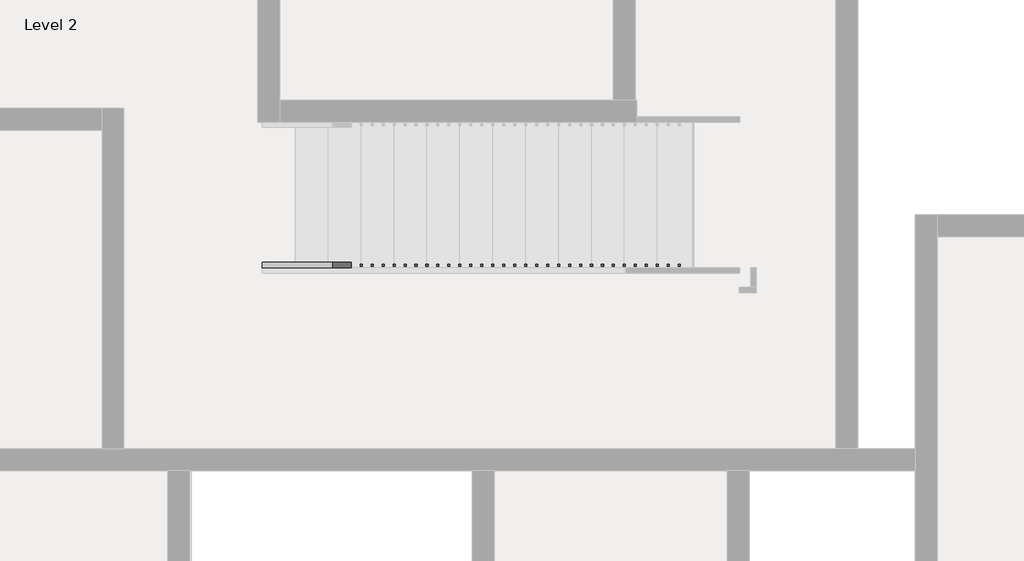
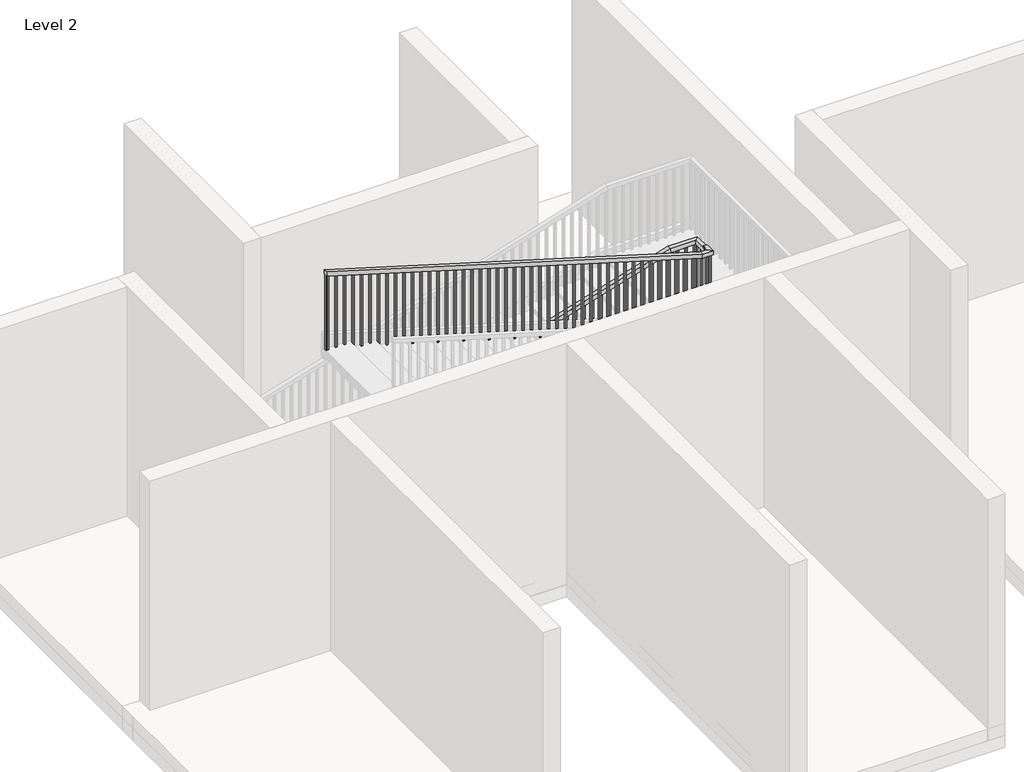
# One storey, part 11 of 14: 1 railing.
"""IFC4 building model written with IfcOpenShell, lengths in millimetres."""

from ifc_helpers import new_model, si_unit, frame, origin, place, context, project, spatial, polyline, outline, extrude, faceted_brep, element, save

model = new_model("IFC4")

# Units and contexts
model_context = context("Model", 3, world=origin())
ifc_project = project(units=[si_unit("LENGTHUNIT", "METRE", prefix="MILLI")], contexts=[model_context])

# Site, building, storey
site = spatial("IfcSite", under=ifc_project)
building = spatial("IfcBuilding", under=site)
storey = spatial("IfcBuildingStorey", under=building, Name="Level 2", Elevation=3048.0)

# Railing
placement = place(None, origin())
element("IfcRailing", 1, ObjectType="Handrail - Rectangular", at=placement, inside=storey, context=model_context, shape_type="SolidModel", body=[
    faceted_brep([(-5254.0891351, 11205.0082924, 4053.84), (-5254.0891351, 11205.0082924, 4000.8032429), (-5254.0891351, 11154.2082924, 4000.8032429), (-5254.0891351, 11154.2082924, 4053.84), (-986.8891351, 11205.0082924, 5334.0), (-979.4332782, 11205.0082924, 5283.2), (-979.4332782, 11154.2082924, 5283.2), (-986.8891351, 11154.2082924, 5334.0), (-631.2891351, 11205.0082924, 5334.0), (-631.2891351, 11205.0082924, 5283.2), (-682.0891351, 11154.2082924, 5283.2), (-682.0891351, 11154.2082924, 5334.0), (-631.2891351, 11001.8082924, 5334.0), (-631.2891351, 10951.0082924, 5283.2), (-682.0891351, 10951.0082924, 5283.2), (-682.0891351, 11001.8082924, 5334.0), (-631.2891351, 11001.8082924, 5356.86), (-631.2891351, 10951.0082924, 5306.06), (-682.0891351, 10951.0082924, 5306.06), (-682.0891351, 11001.8082924, 5356.86), (-631.2891351, 10874.8082924, 5356.86), (-631.2891351, 10874.8082924, 5306.06), (-682.0891351, 10925.6082924, 5306.06), (-682.0891351, 10925.6082924, 5356.86), (-758.2891351, 10874.8082924, 5356.86), (-765.744992, 10874.8082924, 5306.06), (-765.744992, 10925.6082924, 5306.06), (-758.2891351, 10925.6082924, 5356.86), (-5254.0891351, 10874.8082924, 6705.6), (-5254.0891351, 10925.6082924, 6705.6), (-5254.0891351, 10925.6082924, 6652.5632429), (-5254.0891351, 10874.8082924, 6652.5632429)], [[[0, 1, 2, 3]], [[1, 0, 4, 5]], [[2, 1, 5, 6]], [[3, 2, 6, 7]], [[0, 3, 7, 4]], [[5, 4, 8, 9]], [[6, 5, 9, 10]], [[7, 6, 10, 11]], [[4, 7, 11, 8]], [[9, 8, 12, 13]], [[10, 9, 13, 14]], [[11, 10, 14, 15]], [[8, 11, 15, 12]], [[13, 12, 16, 17]], [[14, 13, 17, 18]], [[15, 14, 18, 19]], [[12, 15, 19, 16]], [[17, 16, 20, 21]], [[18, 17, 21, 22]], [[19, 18, 22, 23]], [[16, 19, 23, 20]], [[21, 20, 24, 25]], [[22, 21, 25, 26]], [[23, 22, 26, 27]], [[20, 23, 27, 24]], [[28, 29, 30, 31]], [[25, 24, 28, 31]], [[26, 25, 31, 30]], [[27, 26, 30, 29]], [[24, 27, 29, 28]]]),
    extrude(outline(polyline([(6642.0857429, -5219.1641351), (6647.8007429, -5238.2141351), (5699.76, -5238.2141351), (5699.76, -5219.1641351), (6642.0857429, -5219.1641351)])), frame((0.0, 10890.6832924, 0.0), z_axis=(0.0, 1.0, 0.0), x_axis=(0.0, 0.0, 1.0)), (0.0, 0.0, 1.0), 19.05),
    extrude(outline(polyline([(6611.6057429, -5117.5641351), (6617.3207429, -5136.6141351), (5699.76, -5136.6141351), (5699.76, -5117.5641351), (6611.6057429, -5117.5641351)])), frame((0.0, 10890.6832924, 0.0), z_axis=(0.0, 1.0, 0.0), x_axis=(0.0, 0.0, 1.0)), (0.0, 0.0, 1.0), 19.05),
    extrude(outline(polyline([(6581.1257429, -5015.9641351), (6586.8407429, -5035.0141351), (5699.76, -5035.0141351), (5699.76, -5015.9641351), (6581.1257429, -5015.9641351)])), frame((0.0, 10890.6832924, 0.0), z_axis=(0.0, 1.0, 0.0), x_axis=(0.0, 0.0, 1.0)), (0.0, 0.0, 1.0), 19.05),
    extrude(outline(polyline([(6550.6457429, -4914.3641351), (6556.3607429, -4933.4141351), (5608.32, -4933.4141351), (5608.32, -4914.3641351), (6550.6457429, -4914.3641351)])), frame((0.0, 10890.6832924, 0.0), z_axis=(0.0, 1.0, 0.0), x_axis=(0.0, 0.0, 1.0)), (0.0, 0.0, 1.0), 19.05),
    extrude(outline(polyline([(6520.1657429, -4812.7641351), (6525.8807429, -4831.8141351), (5608.32, -4831.8141351), (5608.32, -4812.7641351), (6520.1657429, -4812.7641351)])), frame((0.0, 10890.6832924, 0.0), z_axis=(0.0, 1.0, 0.0), x_axis=(0.0, 0.0, 1.0)), (0.0, 0.0, 1.0), 19.05),
    extrude(outline(polyline([(6489.6857429, -4711.1641351), (6495.4007429, -4730.2141351), (5608.32, -4730.2141351), (5608.32, -4711.1641351), (6489.6857429, -4711.1641351)])), frame((0.0, 10890.6832924, 0.0), z_axis=(0.0, 1.0, 0.0), x_axis=(0.0, 0.0, 1.0)), (0.0, 0.0, 1.0), 19.05),
    extrude(outline(polyline([(6459.2057429, -4609.5641351), (6464.9207429, -4628.6141351), (5516.88, -4628.6141351), (5516.88, -4609.5641351), (6459.2057429, -4609.5641351)])), frame((0.0, 10890.6832924, 0.0), z_axis=(0.0, 1.0, 0.0), x_axis=(0.0, 0.0, 1.0)), (0.0, 0.0, 1.0), 19.05),
    extrude(outline(polyline([(6428.7257429, -4507.9641351), (6434.4407429, -4527.0141351), (5516.88, -4527.0141351), (5516.88, -4507.9641351), (6428.7257429, -4507.9641351)])), frame((0.0, 10890.6832924, 0.0), z_axis=(0.0, 1.0, 0.0), x_axis=(0.0, 0.0, 1.0)), (0.0, 0.0, 1.0), 19.05),
    extrude(outline(polyline([(6398.2457429, -4406.3641351), (6403.9607429, -4425.4141351), (5516.88, -4425.4141351), (5516.88, -4406.3641351), (6398.2457429, -4406.3641351)])), frame((0.0, 10890.6832924, 0.0), z_axis=(0.0, 1.0, 0.0), x_axis=(0.0, 0.0, 1.0)), (0.0, 0.0, 1.0), 19.05),
    extrude(outline(polyline([(6367.7657429, -4304.7641351), (6373.4807429, -4323.8141351), (5425.44, -4323.8141351), (5425.44, -4304.7641351), (6367.7657429, -4304.7641351)])), frame((0.0, 10890.6832924, 0.0), z_axis=(0.0, 1.0, 0.0), x_axis=(0.0, 0.0, 1.0)), (0.0, 0.0, 1.0), 19.05),
    extrude(outline(polyline([(6337.2857429, -4203.1641351), (6343.0007429, -4222.2141351), (5425.44, -4222.2141351), (5425.44, -4203.1641351), (6337.2857429, -4203.1641351)])), frame((0.0, 10890.6832924, 0.0), z_axis=(0.0, 1.0, 0.0), x_axis=(0.0, 0.0, 1.0)), (0.0, 0.0, 1.0), 19.05),
    extrude(outline(polyline([(6306.8057429, -4101.5641351), (6312.5207429, -4120.6141351), (5425.44, -4120.6141351), (5425.44, -4101.5641351), (6306.8057429, -4101.5641351)])), frame((0.0, 10890.6832924, 0.0), z_axis=(0.0, 1.0, 0.0), x_axis=(0.0, 0.0, 1.0)), (0.0, 0.0, 1.0), 19.05),
    extrude(outline(polyline([(6276.3257429, -3999.9641351), (6282.0407429, -4019.0141351), (5334.0, -4019.0141351), (5334.0, -3999.9641351), (6276.3257429, -3999.9641351)])), frame((0.0, 10890.6832924, 0.0), z_axis=(0.0, 1.0, 0.0), x_axis=(0.0, 0.0, 1.0)), (0.0, 0.0, 1.0), 19.05),
    extrude(outline(polyline([(6245.8457429, -3898.3641351), (6251.5607429, -3917.4141351), (5334.0, -3917.4141351), (5334.0, -3898.3641351), (6245.8457429, -3898.3641351)])), frame((0.0, 10890.6832924, 0.0), z_axis=(0.0, 1.0, 0.0), x_axis=(0.0, 0.0, 1.0)), (0.0, 0.0, 1.0), 19.05),
    extrude(outline(polyline([(6215.3657429, -3796.7641351), (6221.0807429, -3815.8141351), (5334.0, -3815.8141351), (5334.0, -3796.7641351), (6215.3657429, -3796.7641351)])), frame((0.0, 10890.6832924, 0.0), z_axis=(0.0, 1.0, 0.0), x_axis=(0.0, 0.0, 1.0)), (0.0, 0.0, 1.0), 19.05),
    extrude(outline(polyline([(6184.8857429, -3695.1641351), (6190.6007429, -3714.2141351), (5242.56, -3714.2141351), (5242.56, -3695.1641351), (6184.8857429, -3695.1641351)])), frame((0.0, 10890.6832924, 0.0), z_axis=(0.0, 1.0, 0.0), x_axis=(0.0, 0.0, 1.0)), (0.0, 0.0, 1.0), 19.05),
    extrude(outline(polyline([(6154.4057429, -3593.5641351), (6160.1207429, -3612.6141351), (5242.56, -3612.6141351), (5242.56, -3593.5641351), (6154.4057429, -3593.5641351)])), frame((0.0, 10890.6832924, 0.0), z_axis=(0.0, 1.0, 0.0), x_axis=(0.0, 0.0, 1.0)), (0.0, 0.0, 1.0), 19.05),
    extrude(outline(polyline([(6123.9257429, -3491.9641351), (6129.6407429, -3511.0141351), (5242.56, -3511.0141351), (5242.56, -3491.9641351), (6123.9257429, -3491.9641351)])), frame((0.0, 10890.6832924, 0.0), z_axis=(0.0, 1.0, 0.0), x_axis=(0.0, 0.0, 1.0)), (0.0, 0.0, 1.0), 19.05),
    extrude(outline(polyline([(6093.4457429, -3390.3641351), (6099.1607429, -3409.4141351), (5151.12, -3409.4141351), (5151.12, -3390.3641351), (6093.4457429, -3390.3641351)])), frame((0.0, 10890.6832924, 0.0), z_axis=(0.0, 1.0, 0.0), x_axis=(0.0, 0.0, 1.0)), (0.0, 0.0, 1.0), 19.05),
    extrude(outline(polyline([(6062.9657429, -3288.7641351), (6068.6807429, -3307.8141351), (5151.12, -3307.8141351), (5151.12, -3288.7641351), (6062.9657429, -3288.7641351)])), frame((0.0, 10890.6832924, 0.0), z_axis=(0.0, 1.0, 0.0), x_axis=(0.0, 0.0, 1.0)), (0.0, 0.0, 1.0), 19.05),
    extrude(outline(polyline([(6032.4857429, -3187.1641351), (6038.2007429, -3206.2141351), (5151.12, -3206.2141351), (5151.12, -3187.1641351), (6032.4857429, -3187.1641351)])), frame((0.0, 10890.6832924, 0.0), z_axis=(0.0, 1.0, 0.0), x_axis=(0.0, 0.0, 1.0)), (0.0, 0.0, 1.0), 19.05),
    extrude(outline(polyline([(6002.0057429, -3085.5641351), (6007.7207429, -3104.6141351), (5059.68, -3104.6141351), (5059.68, -3085.5641351), (6002.0057429, -3085.5641351)])), frame((0.0, 10890.6832924, 0.0), z_axis=(0.0, 1.0, 0.0), x_axis=(0.0, 0.0, 1.0)), (0.0, 0.0, 1.0), 19.05),
    extrude(outline(polyline([(5971.5257429, -2983.9641351), (5977.2407429, -3003.0141351), (5059.68, -3003.0141351), (5059.68, -2983.9641351), (5971.5257429, -2983.9641351)])), frame((0.0, 10890.6832924, 0.0), z_axis=(0.0, 1.0, 0.0), x_axis=(0.0, 0.0, 1.0)), (0.0, 0.0, 1.0), 19.05),
    extrude(outline(polyline([(5941.0457429, -2882.3641351), (5946.7607429, -2901.4141351), (5059.68, -2901.4141351), (5059.68, -2882.3641351), (5941.0457429, -2882.3641351)])), frame((0.0, 10890.6832924, 0.0), z_axis=(0.0, 1.0, 0.0), x_axis=(0.0, 0.0, 1.0)), (0.0, 0.0, 1.0), 19.05),
    extrude(outline(polyline([(5910.5657429, -2780.7641351), (5916.2807429, -2799.8141351), (4968.24, -2799.8141351), (4968.24, -2780.7641351), (5910.5657429, -2780.7641351)])), frame((0.0, 10890.6832924, 0.0), z_axis=(0.0, 1.0, 0.0), x_axis=(0.0, 0.0, 1.0)), (0.0, 0.0, 1.0), 19.05),
    extrude(outline(polyline([(5880.0857429, -2679.1641351), (5885.8007429, -2698.2141351), (4968.24, -2698.2141351), (4968.24, -2679.1641351), (5880.0857429, -2679.1641351)])), frame((0.0, 10890.6832924, 0.0), z_axis=(0.0, 1.0, 0.0), x_axis=(0.0, 0.0, 1.0)), (0.0, 0.0, 1.0), 19.05),
    extrude(outline(polyline([(5849.6057429, -2577.5641351), (5855.3207429, -2596.6141351), (4968.24, -2596.6141351), (4968.24, -2577.5641351), (5849.6057429, -2577.5641351)])), frame((0.0, 10890.6832924, 0.0), z_axis=(0.0, 1.0, 0.0), x_axis=(0.0, 0.0, 1.0)), (0.0, 0.0, 1.0), 19.05),
    extrude(outline(polyline([(5819.1257429, -2475.9641351), (5824.8407429, -2495.0141351), (4876.8, -2495.0141351), (4876.8, -2475.9641351), (5819.1257429, -2475.9641351)])), frame((0.0, 10890.6832924, 0.0), z_axis=(0.0, 1.0, 0.0), x_axis=(0.0, 0.0, 1.0)), (0.0, 0.0, 1.0), 19.05),
    extrude(outline(polyline([(5788.6457429, -2374.3641351), (5794.3607429, -2393.4141351), (4876.8, -2393.4141351), (4876.8, -2374.3641351), (5788.6457429, -2374.3641351)])), frame((0.0, 10890.6832924, 0.0), z_axis=(0.0, 1.0, 0.0), x_axis=(0.0, 0.0, 1.0)), (0.0, 0.0, 1.0), 19.05),
    extrude(outline(polyline([(5758.1657429, -2272.7641351), (5763.8807429, -2291.8141351), (4876.8, -2291.8141351), (4876.8, -2272.7641351), (5758.1657429, -2272.7641351)])), frame((0.0, 10890.6832924, 0.0), z_axis=(0.0, 1.0, 0.0), x_axis=(0.0, 0.0, 1.0)), (0.0, 0.0, 1.0), 19.05),
    extrude(outline(polyline([(5727.6857429, -2171.1641351), (5733.4007429, -2190.2141351), (4785.36, -2190.2141351), (4785.36, -2171.1641351), (5727.6857429, -2171.1641351)])), frame((0.0, 10890.6832924, 0.0), z_axis=(0.0, 1.0, 0.0), x_axis=(0.0, 0.0, 1.0)), (0.0, 0.0, 1.0), 19.05),
    extrude(outline(polyline([(5697.2057429, -2069.5641351), (5702.9207429, -2088.6141351), (4785.36, -2088.6141351), (4785.36, -2069.5641351), (5697.2057429, -2069.5641351)])), frame((0.0, 10890.6832924, 0.0), z_axis=(0.0, 1.0, 0.0), x_axis=(0.0, 0.0, 1.0)), (0.0, 0.0, 1.0), 19.05),
    extrude(outline(polyline([(5666.7257429, -1967.9641351), (5672.4407429, -1987.0141351), (4785.36, -1987.0141351), (4785.36, -1967.9641351), (5666.7257429, -1967.9641351)])), frame((0.0, 10890.6832924, 0.0), z_axis=(0.0, 1.0, 0.0), x_axis=(0.0, 0.0, 1.0)), (0.0, 0.0, 1.0), 19.05),
    extrude(outline(polyline([(5636.2457429, -1866.3641351), (5641.9607429, -1885.4141351), (4693.92, -1885.4141351), (4693.92, -1866.3641351), (5636.2457429, -1866.3641351)])), frame((0.0, 10890.6832924, 0.0), z_axis=(0.0, 1.0, 0.0), x_axis=(0.0, 0.0, 1.0)), (0.0, 0.0, 1.0), 19.05),
    extrude(outline(polyline([(5605.7657429, -1764.7641351), (5611.4807429, -1783.8141351), (4693.92, -1783.8141351), (4693.92, -1764.7641351), (5605.7657429, -1764.7641351)])), frame((0.0, 10890.6832924, 0.0), z_axis=(0.0, 1.0, 0.0), x_axis=(0.0, 0.0, 1.0)), (0.0, 0.0, 1.0), 19.05),
    extrude(outline(polyline([(5575.2857429, -1663.1641351), (5581.0007429, -1682.2141351), (4693.92, -1682.2141351), (4693.92, -1663.1641351), (5575.2857429, -1663.1641351)])), frame((0.0, 10890.6832924, 0.0), z_axis=(0.0, 1.0, 0.0), x_axis=(0.0, 0.0, 1.0)), (0.0, 0.0, 1.0), 19.05),
    extrude(outline(polyline([(5544.8057429, -1561.5641351), (5550.5207429, -1580.6141351), (4602.48, -1580.6141351), (4602.48, -1561.5641351), (5544.8057429, -1561.5641351)])), frame((0.0, 10890.6832924, 0.0), z_axis=(0.0, 1.0, 0.0), x_axis=(0.0, 0.0, 1.0)), (0.0, 0.0, 1.0), 19.05),
    extrude(outline(polyline([(5514.3257429, -1459.9641351), (5520.0407429, -1479.0141351), (4602.48, -1479.0141351), (4602.48, -1459.9641351), (5514.3257429, -1459.9641351)])), frame((0.0, 10890.6832924, 0.0), z_axis=(0.0, 1.0, 0.0), x_axis=(0.0, 0.0, 1.0)), (0.0, 0.0, 1.0), 19.05),
    extrude(outline(polyline([(5483.8457429, -1358.3641351), (5489.5607429, -1377.4141351), (4602.48, -1377.4141351), (4602.48, -1358.3641351), (5483.8457429, -1358.3641351)])), frame((0.0, 10890.6832924, 0.0), z_axis=(0.0, 1.0, 0.0), x_axis=(0.0, 0.0, 1.0)), (0.0, 0.0, 1.0), 19.05),
    extrude(outline(polyline([(5453.3657429, -1256.7641351), (5459.0807429, -1275.8141351), (4511.04, -1275.8141351), (4511.04, -1256.7641351), (5453.3657429, -1256.7641351)])), frame((0.0, 10890.6832924, 0.0), z_axis=(0.0, 1.0, 0.0), x_axis=(0.0, 0.0, 1.0)), (0.0, 0.0, 1.0), 19.05),
    extrude(outline(polyline([(5422.8857429, -1155.1641351), (5428.6007429, -1174.2141351), (4511.04, -1174.2141351), (4511.04, -1155.1641351), (5422.8857429, -1155.1641351)])), frame((0.0, 10890.6832924, 0.0), z_axis=(0.0, 1.0, 0.0), x_axis=(0.0, 0.0, 1.0)), (0.0, 0.0, 1.0), 19.05),
    extrude(outline(polyline([(5392.4057429, -1053.5641351), (5398.1207429, -1072.6141351), (4511.04, -1072.6141351), (4511.04, -1053.5641351), (5392.4057429, -1053.5641351)])), frame((0.0, 10890.6832924, 0.0), z_axis=(0.0, 1.0, 0.0), x_axis=(0.0, 0.0, 1.0)), (0.0, 0.0, 1.0), 19.05),
    extrude(outline(polyline([(5361.9257429, -951.9641351), (5367.6407429, -971.0141351), (4419.6, -971.0141351), (4419.6, -951.9641351), (5361.9257429, -951.9641351)])), frame((0.0, 10890.6832924, 0.0), z_axis=(0.0, 1.0, 0.0), x_axis=(0.0, 0.0, 1.0)), (0.0, 0.0, 1.0), 19.05),
    extrude(outline(polyline([(5331.4457429, -850.3641351), (5337.1607429, -869.4141351), (4419.6, -869.4141351), (4419.6, -850.3641351), (5331.4457429, -850.3641351)])), frame((0.0, 10890.6832924, 0.0), z_axis=(0.0, 1.0, 0.0), x_axis=(0.0, 0.0, 1.0)), (0.0, 0.0, 1.0), 19.05),
    extrude(outline(polyline([(5300.9657429, -748.7641351), (5306.6807429, -767.8141351), (4419.6, -767.8141351), (4419.6, -748.7641351), (5300.9657429, -748.7641351)])), frame((0.0, 10890.6832924, 0.0), z_axis=(0.0, 1.0, 0.0), x_axis=(0.0, 0.0, 1.0)), (0.0, 0.0, 1.0), 19.05),
    extrude(outline(polyline([(-666.2141351, 10985.9332924), (-647.1641351, 10985.9332924), (-647.1641351, 10966.8832924), (-666.2141351, 10966.8832924), (-666.2141351, 10985.9332924)])), frame((0.0, 0.0, 4419.6), z_axis=(0.0, 0.0, 1.0), x_axis=(1.0, 0.0, 0.0)), (0.0, 0.0, 1.0), 886.46),
    extrude(outline(polyline([(-666.2141351, 11087.5332924), (-647.1641351, 11087.5332924), (-647.1641351, 11068.4832924), (-666.2141351, 11068.4832924), (-666.2141351, 11087.5332924)])), frame((0.0, 0.0, 4419.6), z_axis=(0.0, 0.0, 1.0), x_axis=(1.0, 0.0, 0.0)), (0.0, 0.0, 1.0), 863.6),
    extrude(outline(polyline([(-691.6141351, 11170.0832924), (-691.6141351, 11189.1332924), (-672.5641351, 11189.1332924), (-672.5641351, 11170.0832924), (-691.6141351, 11170.0832924)])), frame((0.0, 0.0, 4419.6), z_axis=(0.0, 0.0, 1.0), x_axis=(1.0, 0.0, 0.0)), (0.0, 0.0, 1.0), 863.6),
    extrude(outline(polyline([(-793.2141351, 11170.0832924), (-793.2141351, 11189.1332924), (-774.1641351, 11189.1332924), (-774.1641351, 11170.0832924), (-793.2141351, 11170.0832924)])), frame((0.0, 0.0, 4419.6), z_axis=(0.0, 0.0, 1.0), x_axis=(1.0, 0.0, 0.0)), (0.0, 0.0, 1.0), 863.6),
    extrude(outline(polyline([(-894.8141351, 11170.0832924), (-894.8141351, 11189.1332924), (-875.7641351, 11189.1332924), (-875.7641351, 11170.0832924), (-894.8141351, 11170.0832924)])), frame((0.0, 0.0, 4419.6), z_axis=(0.0, 0.0, 1.0), x_axis=(1.0, 0.0, 0.0)), (0.0, 0.0, 1.0), 863.6),
    extrude(outline(polyline([(5283.8207429, -977.3641351), (5278.1057429, -996.4141351), (4419.6, -996.4141351), (4419.6, -977.3641351), (5283.8207429, -977.3641351)])), frame((0.0, 11170.0832924, 0.0), z_axis=(0.0, 1.0, 0.0), x_axis=(0.0, 0.0, 1.0)), (0.0, 0.0, 1.0), 19.05),
    extrude(outline(polyline([(5253.3407429, -1078.9641351), (5247.6257429, -1098.0141351), (4328.16, -1098.0141351), (4328.16, -1078.9641351), (5253.3407429, -1078.9641351)])), frame((0.0, 11170.0832924, 0.0), z_axis=(0.0, 1.0, 0.0), x_axis=(0.0, 0.0, 1.0)), (0.0, 0.0, 1.0), 19.05),
    extrude(outline(polyline([(5222.8607429, -1180.5641351), (5217.1457429, -1199.6141351), (4328.16, -1199.6141351), (4328.16, -1180.5641351), (5222.8607429, -1180.5641351)])), frame((0.0, 11170.0832924, 0.0), z_axis=(0.0, 1.0, 0.0), x_axis=(0.0, 0.0, 1.0)), (0.0, 0.0, 1.0), 19.05),
    extrude(outline(polyline([(5192.3807429, -1282.1641351), (5186.6657429, -1301.2141351), (4328.16, -1301.2141351), (4328.16, -1282.1641351), (5192.3807429, -1282.1641351)])), frame((0.0, 11170.0832924, 0.0), z_axis=(0.0, 1.0, 0.0), x_axis=(0.0, 0.0, 1.0)), (0.0, 0.0, 1.0), 19.05),
    extrude(outline(polyline([(5161.9007429, -1383.7641351), (5156.1857429, -1402.8141351), (4236.72, -1402.8141351), (4236.72, -1383.7641351), (5161.9007429, -1383.7641351)])), frame((0.0, 11170.0832924, 0.0), z_axis=(0.0, 1.0, 0.0), x_axis=(0.0, 0.0, 1.0)), (0.0, 0.0, 1.0), 19.05),
    extrude(outline(polyline([(5131.4207429, -1485.3641351), (5125.7057429, -1504.4141351), (4236.72, -1504.4141351), (4236.72, -1485.3641351), (5131.4207429, -1485.3641351)])), frame((0.0, 11170.0832924, 0.0), z_axis=(0.0, 1.0, 0.0), x_axis=(0.0, 0.0, 1.0)), (0.0, 0.0, 1.0), 19.05),
    extrude(outline(polyline([(5100.9407429, -1586.9641351), (5095.2257429, -1606.0141351), (4236.72, -1606.0141351), (4236.72, -1586.9641351), (5100.9407429, -1586.9641351)])), frame((0.0, 11170.0832924, 0.0), z_axis=(0.0, 1.0, 0.0), x_axis=(0.0, 0.0, 1.0)), (0.0, 0.0, 1.0), 19.05),
    extrude(outline(polyline([(5070.4607429, -1688.5641351), (5064.7457429, -1707.6141351), (4145.28, -1707.6141351), (4145.28, -1688.5641351), (5070.4607429, -1688.5641351)])), frame((0.0, 11170.0832924, 0.0), z_axis=(0.0, 1.0, 0.0), x_axis=(0.0, 0.0, 1.0)), (0.0, 0.0, 1.0), 19.05),
    extrude(outline(polyline([(5039.9807429, -1790.1641351), (5034.2657429, -1809.2141351), (4145.28, -1809.2141351), (4145.28, -1790.1641351), (5039.9807429, -1790.1641351)])), frame((0.0, 11170.0832924, 0.0), z_axis=(0.0, 1.0, 0.0), x_axis=(0.0, 0.0, 1.0)), (0.0, 0.0, 1.0), 19.05),
    extrude(outline(polyline([(5009.5007429, -1891.7641351), (5003.7857429, -1910.8141351), (4145.28, -1910.8141351), (4145.28, -1891.7641351), (5009.5007429, -1891.7641351)])), frame((0.0, 11170.0832924, 0.0), z_axis=(0.0, 1.0, 0.0), x_axis=(0.0, 0.0, 1.0)), (0.0, 0.0, 1.0), 19.05),
    extrude(outline(polyline([(4979.0207429, -1993.3641351), (4973.3057429, -2012.4141351), (4053.84, -2012.4141351), (4053.84, -1993.3641351), (4979.0207429, -1993.3641351)])), frame((0.0, 11170.0832924, 0.0), z_axis=(0.0, 1.0, 0.0), x_axis=(0.0, 0.0, 1.0)), (0.0, 0.0, 1.0), 19.05),
    extrude(outline(polyline([(4948.5407429, -2094.9641351), (4942.8257429, -2114.0141351), (4053.84, -2114.0141351), (4053.84, -2094.9641351), (4948.5407429, -2094.9641351)])), frame((0.0, 11170.0832924, 0.0), z_axis=(0.0, 1.0, 0.0), x_axis=(0.0, 0.0, 1.0)), (0.0, 0.0, 1.0), 19.05),
    extrude(outline(polyline([(4918.0607429, -2196.5641351), (4912.3457429, -2215.6141351), (4053.84, -2215.6141351), (4053.84, -2196.5641351), (4918.0607429, -2196.5641351)])), frame((0.0, 11170.0832924, 0.0), z_axis=(0.0, 1.0, 0.0), x_axis=(0.0, 0.0, 1.0)), (0.0, 0.0, 1.0), 19.05),
    extrude(outline(polyline([(4887.5807429, -2298.1641351), (4881.8657429, -2317.2141351), (3962.4, -2317.2141351), (3962.4, -2298.1641351), (4887.5807429, -2298.1641351)])), frame((0.0, 11170.0832924, 0.0), z_axis=(0.0, 1.0, 0.0), x_axis=(0.0, 0.0, 1.0)), (0.0, 0.0, 1.0), 19.05),
    extrude(outline(polyline([(4857.1007429, -2399.7641351), (4851.3857429, -2418.8141351), (3962.4, -2418.8141351), (3962.4, -2399.7641351), (4857.1007429, -2399.7641351)])), frame((0.0, 11170.0832924, 0.0), z_axis=(0.0, 1.0, 0.0), x_axis=(0.0, 0.0, 1.0)), (0.0, 0.0, 1.0), 19.05),
    extrude(outline(polyline([(4826.6207429, -2501.3641351), (4820.9057429, -2520.4141351), (3962.4, -2520.4141351), (3962.4, -2501.3641351), (4826.6207429, -2501.3641351)])), frame((0.0, 11170.0832924, 0.0), z_axis=(0.0, 1.0, 0.0), x_axis=(0.0, 0.0, 1.0)), (0.0, 0.0, 1.0), 19.05),
    extrude(outline(polyline([(4796.1407429, -2602.9641351), (4790.4257429, -2622.0141351), (3870.96, -2622.0141351), (3870.96, -2602.9641351), (4796.1407429, -2602.9641351)])), frame((0.0, 11170.0832924, 0.0), z_axis=(0.0, 1.0, 0.0), x_axis=(0.0, 0.0, 1.0)), (0.0, 0.0, 1.0), 19.05),
    extrude(outline(polyline([(4765.6607429, -2704.5641351), (4759.9457429, -2723.6141351), (3870.96, -2723.6141351), (3870.96, -2704.5641351), (4765.6607429, -2704.5641351)])), frame((0.0, 11170.0832924, 0.0), z_axis=(0.0, 1.0, 0.0), x_axis=(0.0, 0.0, 1.0)), (0.0, 0.0, 1.0), 19.05),
    extrude(outline(polyline([(4735.1807429, -2806.1641351), (4729.4657429, -2825.2141351), (3870.96, -2825.2141351), (3870.96, -2806.1641351), (4735.1807429, -2806.1641351)])), frame((0.0, 11170.0832924, 0.0), z_axis=(0.0, 1.0, 0.0), x_axis=(0.0, 0.0, 1.0)), (0.0, 0.0, 1.0), 19.05),
    extrude(outline(polyline([(4704.7007429, -2907.7641351), (4698.9857429, -2926.8141351), (3779.52, -2926.8141351), (3779.52, -2907.7641351), (4704.7007429, -2907.7641351)])), frame((0.0, 11170.0832924, 0.0), z_axis=(0.0, 1.0, 0.0), x_axis=(0.0, 0.0, 1.0)), (0.0, 0.0, 1.0), 19.05),
    extrude(outline(polyline([(4674.2207429, -3009.3641351), (4668.5057429, -3028.4141351), (3779.52, -3028.4141351), (3779.52, -3009.3641351), (4674.2207429, -3009.3641351)])), frame((0.0, 11170.0832924, 0.0), z_axis=(0.0, 1.0, 0.0), x_axis=(0.0, 0.0, 1.0)), (0.0, 0.0, 1.0), 19.05),
    extrude(outline(polyline([(4643.7407429, -3110.9641351), (4638.0257429, -3130.0141351), (3779.52, -3130.0141351), (3779.52, -3110.9641351), (4643.7407429, -3110.9641351)])), frame((0.0, 11170.0832924, 0.0), z_axis=(0.0, 1.0, 0.0), x_axis=(0.0, 0.0, 1.0)), (0.0, 0.0, 1.0), 19.05),
    extrude(outline(polyline([(4613.2607429, -3212.5641351), (4607.5457429, -3231.6141351), (3688.08, -3231.6141351), (3688.08, -3212.5641351), (4613.2607429, -3212.5641351)])), frame((0.0, 11170.0832924, 0.0), z_axis=(0.0, 1.0, 0.0), x_axis=(0.0, 0.0, 1.0)), (0.0, 0.0, 1.0), 19.05),
    extrude(outline(polyline([(4582.7807429, -3314.1641351), (4577.0657429, -3333.2141351), (3688.08, -3333.2141351), (3688.08, -3314.1641351), (4582.7807429, -3314.1641351)])), frame((0.0, 11170.0832924, 0.0), z_axis=(0.0, 1.0, 0.0), x_axis=(0.0, 0.0, 1.0)), (0.0, 0.0, 1.0), 19.05),
    extrude(outline(polyline([(4552.3007429, -3415.7641351), (4546.5857429, -3434.8141351), (3688.08, -3434.8141351), (3688.08, -3415.7641351), (4552.3007429, -3415.7641351)])), frame((0.0, 11170.0832924, 0.0), z_axis=(0.0, 1.0, 0.0), x_axis=(0.0, 0.0, 1.0)), (0.0, 0.0, 1.0), 19.05),
    extrude(outline(polyline([(4521.8207429, -3517.3641351), (4516.1057429, -3536.4141351), (3596.64, -3536.4141351), (3596.64, -3517.3641351), (4521.8207429, -3517.3641351)])), frame((0.0, 11170.0832924, 0.0), z_axis=(0.0, 1.0, 0.0), x_axis=(0.0, 0.0, 1.0)), (0.0, 0.0, 1.0), 19.05),
    extrude(outline(polyline([(4491.3407429, -3618.9641351), (4485.6257429, -3638.0141351), (3596.64, -3638.0141351), (3596.64, -3618.9641351), (4491.3407429, -3618.9641351)])), frame((0.0, 11170.0832924, 0.0), z_axis=(0.0, 1.0, 0.0), x_axis=(0.0, 0.0, 1.0)), (0.0, 0.0, 1.0), 19.05),
    extrude(outline(polyline([(4460.8607429, -3720.5641351), (4455.1457429, -3739.6141351), (3596.64, -3739.6141351), (3596.64, -3720.5641351), (4460.8607429, -3720.5641351)])), frame((0.0, 11170.0832924, 0.0), z_axis=(0.0, 1.0, 0.0), x_axis=(0.0, 0.0, 1.0)), (0.0, 0.0, 1.0), 19.05),
    extrude(outline(polyline([(4430.3807429, -3822.1641351), (4424.6657429, -3841.2141351), (3505.2, -3841.2141351), (3505.2, -3822.1641351), (4430.3807429, -3822.1641351)])), frame((0.0, 11170.0832924, 0.0), z_axis=(0.0, 1.0, 0.0), x_axis=(0.0, 0.0, 1.0)), (0.0, 0.0, 1.0), 19.05),
    extrude(outline(polyline([(4399.9007429, -3923.7641351), (4394.1857429, -3942.8141351), (3505.2, -3942.8141351), (3505.2, -3923.7641351), (4399.9007429, -3923.7641351)])), frame((0.0, 11170.0832924, 0.0), z_axis=(0.0, 1.0, 0.0), x_axis=(0.0, 0.0, 1.0)), (0.0, 0.0, 1.0), 19.05),
    extrude(outline(polyline([(4369.4207429, -4025.3641351), (4363.7057429, -4044.4141351), (3505.2, -4044.4141351), (3505.2, -4025.3641351), (4369.4207429, -4025.3641351)])), frame((0.0, 11170.0832924, 0.0), z_axis=(0.0, 1.0, 0.0), x_axis=(0.0, 0.0, 1.0)), (0.0, 0.0, 1.0), 19.05),
    extrude(outline(polyline([(4338.9407429, -4126.9641351), (4333.2257429, -4146.0141351), (3413.76, -4146.0141351), (3413.76, -4126.9641351), (4338.9407429, -4126.9641351)])), frame((0.0, 11170.0832924, 0.0), z_axis=(0.0, 1.0, 0.0), x_axis=(0.0, 0.0, 1.0)), (0.0, 0.0, 1.0), 19.05),
    extrude(outline(polyline([(4308.4607429, -4228.5641351), (4302.7457429, -4247.6141351), (3413.76, -4247.6141351), (3413.76, -4228.5641351), (4308.4607429, -4228.5641351)])), frame((0.0, 11170.0832924, 0.0), z_axis=(0.0, 1.0, 0.0), x_axis=(0.0, 0.0, 1.0)), (0.0, 0.0, 1.0), 19.05),
    extrude(outline(polyline([(4277.9807429, -4330.1641351), (4272.2657429, -4349.2141351), (3413.76, -4349.2141351), (3413.76, -4330.1641351), (4277.9807429, -4330.1641351)])), frame((0.0, 11170.0832924, 0.0), z_axis=(0.0, 1.0, 0.0), x_axis=(0.0, 0.0, 1.0)), (0.0, 0.0, 1.0), 19.05),
    extrude(outline(polyline([(4247.5007429, -4431.7641351), (4241.7857429, -4450.8141351), (3322.32, -4450.8141351), (3322.32, -4431.7641351), (4247.5007429, -4431.7641351)])), frame((0.0, 11170.0832924, 0.0), z_axis=(0.0, 1.0, 0.0), x_axis=(0.0, 0.0, 1.0)), (0.0, 0.0, 1.0), 19.05),
    extrude(outline(polyline([(4217.0207429, -4533.3641351), (4211.3057429, -4552.4141351), (3322.32, -4552.4141351), (3322.32, -4533.3641351), (4217.0207429, -4533.3641351)])), frame((0.0, 11170.0832924, 0.0), z_axis=(0.0, 1.0, 0.0), x_axis=(0.0, 0.0, 1.0)), (0.0, 0.0, 1.0), 19.05),
    extrude(outline(polyline([(4186.5407429, -4634.9641351), (4180.8257429, -4654.0141351), (3322.32, -4654.0141351), (3322.32, -4634.9641351), (4186.5407429, -4634.9641351)])), frame((0.0, 11170.0832924, 0.0), z_axis=(0.0, 1.0, 0.0), x_axis=(0.0, 0.0, 1.0)), (0.0, 0.0, 1.0), 19.05),
    extrude(outline(polyline([(4156.0607429, -4736.5641351), (4150.3457429, -4755.6141351), (3230.88, -4755.6141351), (3230.88, -4736.5641351), (4156.0607429, -4736.5641351)])), frame((0.0, 11170.0832924, 0.0), z_axis=(0.0, 1.0, 0.0), x_axis=(0.0, 0.0, 1.0)), (0.0, 0.0, 1.0), 19.05),
    extrude(outline(polyline([(4125.5807429, -4838.1641351), (4119.8657429, -4857.2141351), (3230.88, -4857.2141351), (3230.88, -4838.1641351), (4125.5807429, -4838.1641351)])), frame((0.0, 11170.0832924, 0.0), z_axis=(0.0, 1.0, 0.0), x_axis=(0.0, 0.0, 1.0)), (0.0, 0.0, 1.0), 19.05),
    extrude(outline(polyline([(4095.1007429, -4939.7641351), (4089.3857429, -4958.8141351), (3230.88, -4958.8141351), (3230.88, -4939.7641351), (4095.1007429, -4939.7641351)])), frame((0.0, 11170.0832924, 0.0), z_axis=(0.0, 1.0, 0.0), x_axis=(0.0, 0.0, 1.0)), (0.0, 0.0, 1.0), 19.05),
    extrude(outline(polyline([(4064.6207429, -5041.3641351), (4058.9057429, -5060.4141351), (3139.44, -5060.4141351), (3139.44, -5041.3641351), (4064.6207429, -5041.3641351)])), frame((0.0, 11170.0832924, 0.0), z_axis=(0.0, 1.0, 0.0), x_axis=(0.0, 0.0, 1.0)), (0.0, 0.0, 1.0), 19.05),
    extrude(outline(polyline([(4034.1407429, -5142.9641351), (4028.4257429, -5162.0141351), (3139.44, -5162.0141351), (3139.44, -5142.9641351), (4034.1407429, -5142.9641351)])), frame((0.0, 11170.0832924, 0.0), z_axis=(0.0, 1.0, 0.0), x_axis=(0.0, 0.0, 1.0)), (0.0, 0.0, 1.0), 19.05),
    extrude(outline(polyline([(-666.2141351, 10909.7332924), (-647.1641351, 10909.7332924), (-647.1641351, 10890.6832924), (-666.2141351, 10890.6832924), (-666.2141351, 10909.7332924)])), frame((0.0, 0.0, 4419.6), z_axis=(0.0, 0.0, 1.0), x_axis=(1.0, 0.0, 0.0)), (0.0, 0.0, 1.0), 886.46),
    extrude(outline(polyline([(-666.2141351, 11170.0832924), (-666.2141351, 11189.1332924), (-647.1641351, 11189.1332924), (-647.1641351, 11170.0832924), (-666.2141351, 11170.0832924)])), frame((0.0, 0.0, 4419.6), z_axis=(0.0, 0.0, 1.0), x_axis=(1.0, 0.0, 0.0)), (0.0, 0.0, 1.0), 863.6),
    extrude(outline(polyline([(6646.8482429, -5235.0391351), (6652.5632429, -5254.0891351), (5699.76, -5254.0891351), (5699.76, -5235.0391351), (6646.8482429, -5235.0391351)])), frame((0.0, 10890.6832924, 0.0), z_axis=(0.0, 1.0, 0.0), x_axis=(0.0, 0.0, 1.0)), (0.0, 0.0, 1.0), 19.05),
    extrude(outline(polyline([(4006.5182429, -5235.0391351), (4000.8032429, -5254.0891351), (3139.44, -5254.0891351), (3139.44, -5235.0391351), (4006.5182429, -5235.0391351)])), frame((0.0, 11170.0832924, 0.0), z_axis=(0.0, 1.0, 0.0), x_axis=(0.0, 0.0, 1.0)), (0.0, 0.0, 1.0), 19.05),
])

save(model, "model.ifc")

# Revit data of these elements
# Type "Handrail - Rectangular"
#   Assembly Code = "C2010400"
#   built-in parameter 1008612 = 0.0416667 (stored number, unit not read)
#   built-in parameter 1008611 = 0.0416667 (stored number, unit not read)
#   built-in parameter 1008609 = 0.333333 (stored number, unit not read)
#   built-in parameter 1008604 = 0.166667 (stored number, unit not read)
#   built-in parameter 1008603 = 0.166667 (stored number, unit not read)
#   Railing Height = 3' - 0"
#   built-in parameter 1008630 = 2
#   built-in parameter 1008610 = 2
#   built-in parameter 1008618 = Baluster - Square : 3/4"
# Element 1 (IfcRailing, "Handrail - Rectangular")
#   Phase Created = New Construction
